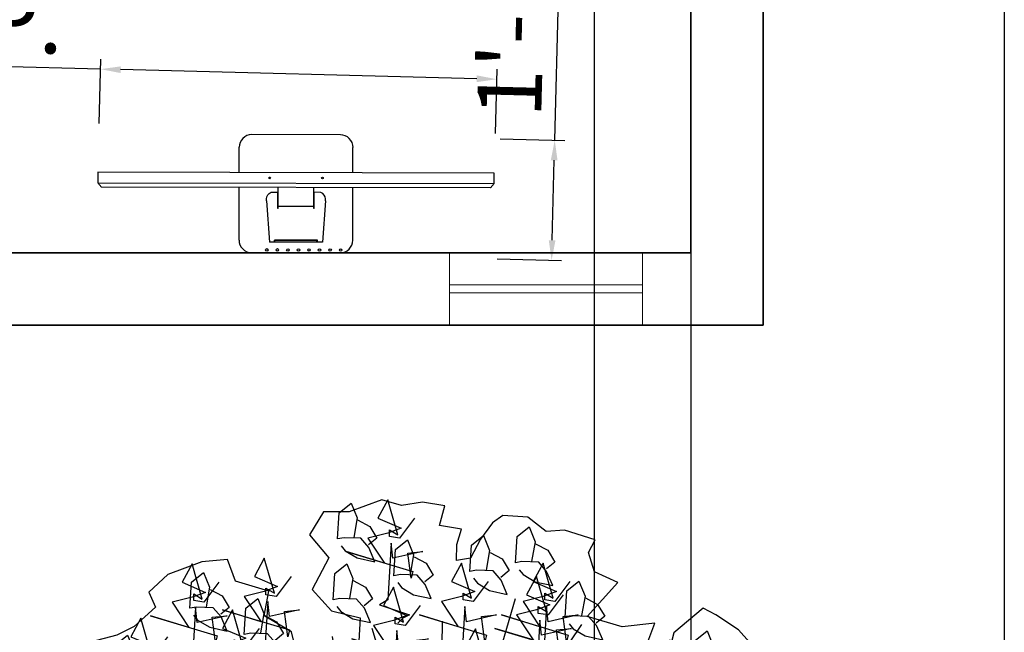
# Model space of a CAD drawing. Units: inches. Extents: x 3394 to 4794, y 965 to 1718.
# Tile 4 of 15: x 3818 to 3941, y 1160 to 1237. Entities that reach past the tile are written whole.
import ezdxf

# ---------------------------------------------------------------- set-up
doc = ezdxf.new("R2010")
doc.units = ezdxf.units.IN
for name, color, linetype, lineweight in [('A-ANNO-DIMS', 2, 'Continuous', 13), ('A-EQPM', 8, 'Continuous', 18), ('A-GLAZ', 4, 'Continuous', 18), ('A-WALL', 7, 'Continuous', 35), ('C-PROP', 7, 'Continuous', 25), ('CAY', 94, 'Continuous', 13)]:
    doc.layers.add(name, color=color, linetype=linetype, lineweight=lineweight)
for name, color, linetype in [('ARBOL', 74, 'Continuous'), ('TALLO', 36, 'Continuous'), ('window', 130, 'Continuous')]:
    doc.layers.add(name, color=color, linetype=linetype)
doc.styles.get("Standard").update_dxf_attribs({"font": 'arial.ttf'})
doc.dimstyles.new('ISO-25', dxfattribs={"dimtxt": 8, "dimasz": 2.5, "dimexe": 1.25, "dimexo": 0.625, "dimtad": 1, "dimlunit": 3, "dimtxsty": 'Standard', "dimcen": 2.5, "dimadec": 0, "dimazin": 0, "dimtfac": 1, "dimtmove": 0, "dimatfit": 3, "dimfxl": 1, "dimarcsym": 0})

# ---------------------------------------------------------------- blocks, each defined once
blk = doc.blocks.new('TV')
at = {"color": 0}
for p, q in [((3967.269, 1784.848), (3967.048, 1784.654)), ((3967.765, 1763.677), (3967.535, 1763.861))]:
    blk.add_line(p, q, dxfattribs=at)
at = {"layer": 'window'}
for p, q in [((3967.535, 1763.861), (3967.048, 1784.654)), ((3964.405, 1777.232), (3967.221, 1777.298)), ((3968.009, 1777.316), (3969.36, 1777.348)), ((3966.535, 1775.819), (3964.331, 1775.605)), ((3964.337, 1775.337), (3964.45, 1775.34)), ((3964.337, 1775.315), (3964.428, 1775.317)), ((3966.143, 1775.199), (3967.01, 1775.22)), ((3966.144, 1775.177), (3966.143, 1775.199)), ((3966.144, 1775.177), (3967.27, 1775.203)), ((3966.3, 1773.288), (3966.256, 1775.179)), ((3964.39, 1773.063), (3964.48, 1773.065)), ((3966.188, 1773.285), (3967.314, 1773.311)), ((3966.188, 1773.262), (3966.188, 1773.285)), ((3966.188, 1773.262), (3967.055, 1773.283)), ((3964.391, 1773.04), (3964.503, 1773.043)), ((3966.608, 1772.662), (3964.397, 1772.772)), ((3964.548, 1771.151), (3967.363, 1771.217)), ((3968.151, 1771.235), (3969.503, 1771.267))]:
    blk.add_line(p, q, dxfattribs=at)
for points in [[(3968.328, 1763.69), (3967.832, 1784.861), (3967.269, 1784.848), (3967.765, 1763.677), (3968.328, 1763.69)], [(3963.856, 1771.811), (3963.745, 1776.54)], [(3970.163, 1771.958), (3970.052, 1776.688)], [(3964.397, 1772.772), (3964.331, 1775.605)], [(3964.48, 1773.065), (3964.428, 1775.317)], [(3964.503, 1773.043), (3964.45, 1775.34)]]:
    blk.add_lwpolyline(points, dxfattribs=at)
for points in [[(3966.535, 1775.819, -0.263666), (3966.933, 1775.689), (3967.001, 1775.572), (3967.01, 1775.22)], [(3966.608, 1772.662, 0.263666), (3967, 1772.811), (3967.063, 1772.93), (3967.055, 1773.283)]]:
    blk.add_lwpolyline(points, format="xyb", dxfattribs=at)
for centre, radius in [((3963.914, 1775.731), 0.0679), ((3967.766, 1775.678), 0.0451), ((3963.927, 1775.168), 0.0679), ((3963.94, 1774.605), 0.0679), ((3963.953, 1774.042), 0.0679), ((3963.966, 1773.478), 0.0679), ((3963.979, 1772.915), 0.0679), ((3967.832, 1772.86), 0.0451), ((3963.993, 1772.352), 0.0679), ((3964.006, 1771.789), 0.0679)]:
    blk.add_circle(centre, radius, dxfattribs=at)
for centre, start, end in [((3969.376, 1776.672), 1.3414, 91.3414), ((3964.421, 1776.556), 91.3414, 181.3414), ((3964.532, 1771.826), 181.3414, 271.3414), ((3969.487, 1771.942), 271.3414, 1.3414)]:
    blk.add_arc(centre, 0.676, start, end, dxfattribs=at)
blk = doc.blocks.new('fresno')
at = {"layer": 'ARBOL'}
for p, q in [((2.96, 0.991), (3.575, 1.984)), ((-3.638, 1.194), (-4.164, 1.76)), ((-1.151, -0.932), (-1.99, -1.556)), ((-0.974, -3.757), (-1.31, -4.423))]:
    blk.add_line(p, q, dxfattribs=at)
blk.add_lwpolyline([(0.823, 4.745), (0.566, 4.764), (0.459, 4.687), (0.336, 4.518), (0.233, 4.322), (0.087, 4.298), (0.091, 4.464), (0.14, 4.621), (-0.09, 4.659), (-0.033, 4.863), (-0.264, 4.901), (-0.483, 4.866), (-0.686, 4.924), (-1.021, 4.801), (-1.288, 4.8), (-1.431, 4.563), (-1.234, 4.327), (-1.406, 4), (-1.205, 3.778), (-0.909, 3.705), (-0.931, 3.283), (-1.122, 2.983), (-1.491, 3.043), (-1.619, 3.562), (-1.9, 3.727), (-1.851, 3.982), (-2.197, 4.084), (-2.278, 4.31), (-2.543, 4.283), (-2.896, 4.152), (-3.091, 3.971), (-3.022, 3.817), (-3.244, 3.617), (-3.424, 3.528), (-3.697, 3.455), (-3.946, 3.236), (-3.922, 3.09), (-3.94, 2.548), (-3.617, 2.495), (-3.927, 2.19), (-4.062, 2.379), (-4.443, 2.512), (-4.546, 2.316), (-4.73, 2.062), (-4.767, 1.832), (-4.671, 1.698), (-4.486, 1.667), (-4.693, 1.559), (-4.854, 1.444), (-4.934, 1.102), (-5.037, 0.905), (-5.175, 0.644), (-5.166, 0.406), (-5.024, 0.264), (-4.781, 0.153), (-4.363, 0.249), (-4.014, 0.215), (-3.783, 0.177), (-3.46, 0.124), (-3.733, 0.051), (-4.132, -0.073), (-4.404, -0.146), (-4.639, 0.011), (-4.977, -0.028), (-5.172, -0.209), (-5.113, -0.574), (-4.921, -0.843), (-4.951, -1.027), (-5.012, -1.112), (-4.95, -1.311), (-4.83, -1.592), (-4.676, -1.807), (-4.518, -1.856), (-4.529, -2.068), (-4.417, -2.394), (-4.236, -2.59), (-4.143, -2.605), (-3.967, -2.397), (-3.703, -2.37), (-3.339, -2.027), (-3.032, -1.889), (-3.169, -2.15), (-3.115, -2.396), (-3.376, -2.542), (-3.552, -2.466), (-3.909, -2.762), (-4.077, -2.924), (-3.804, -3.135), (-3.592, -3.43), (-3.461, -3.499), (-3.253, -3.676), (-2.953, -3.867), (-2.792, -3.752), (-2.642, -3.848), (-2.572, -4.001), (-2.323, -4.066), (-2.18, -4.208), (-1.926, -4.392), (-1.58, -4.591), (-1.288, -4.545), (-1.027, -4.683), (-0.788, -4.675), (-0.531, -4.693), (-0.382, -4.505), (-0.29, -4.236), (-0.66, -3.891), (-0.588, -3.595), (-0.374, -3.441), (-0.267, -3.079), (-0.368, -2.541), (-0.208, -2.426), (-0.099, -2.633), (-0.087, -2.991), (0.071, -3.04), (0.129, -3.405), (-0.185, -3.59), (-0.119, -3.909), (0.055, -4.151), (0.136, -4.377), (0.456, -4.596), (0.828, -4.491), (1.227, -4.368), (1.461, -4.241), (1.583, -4.071), (1.748, -4.075), (1.86, -4.117), (2.101, -3.944), (2.308, -3.836), (2.925, -3.393), (3.101, -3.185), (2.74, -3.078), (2.812, -2.782), (2.769, -2.61), (3.015, -2.555), (3.012, -2.721), (3.254, -2.832), (3.546, -2.785), (3.752, -2.393), (3.882, -2.177), (3.92, -1.947), (4.069, -1.758), (4.214, -1.451), (4.144, -1.297), (4.021, -1.182), (4.182, -1.067), (4.304, -0.897), (4.464, -0.497), (4.429, -0.279), (4.406, -0.133), (3.964, -0.083), (3.074, -0.315), (2.582, -0.424), (2.217, -0.197), (2.136, 0.029), (2.462, 0.141), (2.628, -0.147), (3.012, -0.116), (3.249, 0.177), (3.602, 0.308), (3.701, 0.623), (4.089, 0.535), (4.404, 0.436), (4.464, 0.805), (4.272, 1.074), (4.267, 1.193), (4.336, 1.324), (4.243, 1.623), (4.092, 2.003), (3.769, 2.057), (3.485, 2.056), (3.642, 2.291), (3.88, 2.299), (3.71, 2.706), (3.563, 2.967), (3.201, 3.358), (3.001, 3.581), (2.766, 3.738), (2.635, 3.807), (2.332, 3.549), (2.268, 3.299), (2.052, 3.429), (2.136, 3.652), (1.798, 3.613), (1.437, 3.72), (1.755, 4.071), (1.513, 4.182), (1.451, 4.381), (1.519, 4.512), (1.204, 4.611), (1.012, 4.596)], close=True, dxfattribs=at)
for points in [[(-1.104, 4.45), (-1.063, 4.399), (-0.939, 4.325), (-0.757, 4.285), (-0.82, 4.431), (-0.903, 4.527), (-1.075, 4.533), (-1.143, 4.521), (-1.126, 4.792), (-1.002, 4.891), (-0.939, 4.738), (-0.975, 4.535)], [(-0.346, 4.735), (-0.501, 4.528), (-0.605, 4.545), (-0.605, 4.614), (-0.519, 4.563), (-0.622, 4.925), (-0.726, 4.735), (-0.484, 4.632), (-0.622, 4.58), (-0.829, 4.528), (-0.657, 4.27), (-1.053, 4.39), (-0.363, 4.183), (-0.381, 4.114), (-0.415, 4.373), (-0.26, 4.39), (-0.57, 4.321), (-0.588, 4.476), (-0.622, 3.89), (-0.708, 3.839), (-0.398, 3.735), (-0.467, 3.701), (-0.519, 3.649)], [(-0.935, 4.717), (-0.809, 4.65), (-0.736, 4.529), (-0.824, 4.459)], [(0.734, 4.203), (0.775, 4.152), (0.9, 4.078), (1.082, 4.038), (1.018, 4.185), (0.936, 4.281), (0.763, 4.287), (0.696, 4.274), (0.712, 4.546), (0.837, 4.645), (0.899, 4.491), (0.863, 4.289)], [(-0.521, 4.069), (-0.48, 4.018), (-0.356, 3.944), (-0.174, 3.904), (-0.237, 4.051), (-0.32, 4.146), (-0.492, 4.152), (-0.56, 4.14), (-0.543, 4.411), (-0.419, 4.511), (-0.356, 4.357), (-0.392, 4.154)], [(0.263, 4.114), (0.304, 4.063), (0.429, 3.989), (0.611, 3.948), (0.547, 4.095), (0.465, 4.191), (0.293, 4.197), (0.225, 4.185), (0.242, 4.456), (0.366, 4.555), (0.428, 4.402), (0.393, 4.199)], [(0.433, 4.381), (0.558, 4.314), (0.631, 4.193), (0.544, 4.122)], [(0.904, 4.471), (1.029, 4.404), (1.102, 4.282), (1.015, 4.212)], [(-1.623, 4.132), (-1.778, 3.925), (-1.882, 3.942), (-1.882, 4.011), (-1.795, 3.959), (-1.899, 4.321), (-2.002, 4.132), (-1.761, 4.028), (-1.899, 3.977), (-2.106, 3.925), (-1.933, 3.666), (-2.33, 3.787), (-1.64, 3.58), (-1.657, 3.511), (-1.692, 3.77), (-1.537, 3.787), (-1.847, 3.718), (-1.864, 3.873), (-1.899, 3.287), (-1.985, 3.235), (-1.675, 3.132), (-1.744, 3.097), (-1.795, 3.046)], [(-0.352, 4.337), (-0.226, 4.269), (-0.153, 4.148), (-0.241, 4.078)], [(-2.368, 4.073), (-2.523, 3.866), (-2.627, 3.883), (-2.627, 3.952), (-2.541, 3.9), (-2.644, 4.262), (-2.748, 4.073), (-2.506, 3.969), (-2.644, 3.918), (-2.851, 3.866), (-2.679, 3.607), (-3.075, 3.728), (-2.385, 3.521), (-2.403, 3.452), (-2.437, 3.711), (-2.282, 3.728), (-2.592, 3.659), (-2.61, 3.814), (-2.644, 3.228), (-2.73, 3.176), (-2.42, 3.073), (-2.489, 3.038), (-2.541, 2.987)], [(-2.629, 3.733), (-2.588, 3.682), (-2.463, 3.608), (-2.281, 3.568), (-2.345, 3.715), (-2.427, 3.81), (-2.6, 3.816), (-2.667, 3.804), (-2.651, 4.075), (-2.526, 4.175), (-2.464, 4.021), (-2.5, 3.818)], [(-1.149, 3.822), (-1.108, 3.771), (-0.983, 3.697), (-0.802, 3.657), (-0.865, 3.804), (-0.948, 3.9), (-1.12, 3.906), (-1.188, 3.893), (-1.171, 4.165), (-1.047, 4.264), (-0.984, 4.111), (-1.02, 3.908)], [(0.413, 4.08), (0.258, 3.873), (0.154, 3.89), (0.154, 3.959), (0.241, 3.908), (0.137, 4.27), (0.034, 4.08), (0.275, 3.977), (0.137, 3.925), (-0.07, 3.873), (0.103, 3.614), (-0.294, 3.735), (0.396, 3.528), (0.379, 3.459), (0.344, 3.718), (0.499, 3.735), (0.189, 3.666), (0.172, 3.821), (0.137, 3.235), (0.051, 3.183), (0.361, 3.08), (0.292, 3.046), (0.241, 2.994)], [(1.259, 4.08), (1.103, 3.873), (1, 3.89), (1, 3.959), (1.086, 3.908), (0.982, 4.27), (0.879, 4.08), (1.12, 3.977), (0.982, 3.925), (0.775, 3.873), (0.948, 3.614), (0.551, 3.735), (1.241, 3.528), (1.224, 3.459), (1.189, 3.718), (1.345, 3.735), (1.034, 3.666), (1.017, 3.821), (0.982, 3.235), (0.896, 3.183), (1.207, 3.08), (1.138, 3.046), (1.086, 2.994)], [(-0.98, 4.09), (-0.854, 4.023), (-0.781, 3.901), (-0.869, 3.831)], [(1.189, 3.942), (1.034, 3.735), (0.931, 3.752), (0.931, 3.821), (1.017, 3.77), (0.913, 4.132), (0.81, 3.942), (1.051, 3.839), (0.913, 3.787), (0.706, 3.735), (0.879, 3.477), (0.482, 3.597), (1.172, 3.39), (1.155, 3.321), (1.12, 3.58), (1.276, 3.597), (0.965, 3.528), (0.948, 3.683), (0.913, 3.097), (0.827, 3.046), (1.138, 2.942), (1.069, 2.908), (1.017, 2.856)], [(1.25, 3.643), (1.291, 3.592), (1.416, 3.518), (1.597, 3.478), (1.534, 3.625), (1.451, 3.721), (1.279, 3.727), (1.211, 3.714), (1.228, 3.985), (1.352, 4.085), (1.415, 3.931), (1.379, 3.729)], [(-2.459, 4), (-2.334, 3.933), (-2.261, 3.812), (-2.348, 3.742)], [(-0.287, 3.833), (-0.442, 3.626), (-0.546, 3.643), (-0.546, 3.712), (-0.46, 3.661), (-0.563, 4.023), (-0.667, 3.833), (-0.425, 3.73), (-0.563, 3.678), (-0.77, 3.626), (-0.598, 3.367), (-0.995, 3.488), (-0.304, 3.281), (-0.322, 3.212), (-0.356, 3.471), (-0.201, 3.488), (-0.511, 3.419), (-0.529, 3.574), (-0.563, 2.988), (-0.649, 2.936), (-0.339, 2.833), (-0.408, 2.799), (-0.46, 2.747)], [(-2.068, 3.464), (-2.027, 3.413), (-1.903, 3.339), (-1.721, 3.299), (-1.784, 3.446), (-1.867, 3.542), (-2.039, 3.547), (-2.107, 3.535), (-2.09, 3.806), (-1.966, 3.906), (-1.903, 3.752), (-1.939, 3.55)], [(0.837, 2.414), (0.533, 3.352), (0.697, 3.906)], [(1.419, 3.911), (1.545, 3.844), (1.618, 3.722), (1.53, 3.652)], [(-1.951, 3.597), (-2.106, 3.39), (-2.209, 3.408), (-2.209, 3.477), (-2.123, 3.425), (-2.227, 3.787), (-2.33, 3.597), (-2.089, 3.494), (-2.227, 3.442), (-2.434, 3.39), (-2.261, 3.132), (-2.658, 3.252), (-1.968, 3.046), (-1.985, 2.977), (-2.02, 3.235), (-1.864, 3.252), (-2.175, 3.183), (-2.192, 3.339), (-2.227, 2.752), (-2.313, 2.701), (-2.002, 2.597), (-2.071, 2.563), (-2.123, 2.511)], [(-2.898, 3.511), (-3.053, 3.304), (-3.157, 3.321), (-3.157, 3.39), (-3.071, 3.339), (-3.174, 3.701), (-3.278, 3.511), (-3.036, 3.408), (-3.174, 3.356), (-3.381, 3.304), (-3.209, 3.046), (-3.605, 3.166), (-2.915, 2.959), (-2.932, 2.89), (-2.967, 3.149), (-2.812, 3.166), (-3.122, 3.097), (-3.14, 3.253), (-3.174, 2.666), (-3.26, 2.615), (-2.95, 2.511), (-3.019, 2.477), (-3.071, 2.425)], [(-1.899, 3.732), (-1.773, 3.664), (-1.7, 3.543), (-1.788, 3.473)], [(-0.063, 3.671), (-0.069, 3.151), (-0.364, 2.965), (-0.319, 2.449)], [(-0.358, 2.895), (-0.615, 3.037), (-0.783, 3.596)], [(0.558, 3.402), (0.403, 3.195), (0.299, 3.212), (0.299, 3.281), (0.386, 3.23), (0.282, 3.592), (0.179, 3.402), (0.42, 3.299), (0.282, 3.247), (0.075, 3.195), (0.248, 2.936), (-0.149, 3.057), (0.541, 2.85), (0.524, 2.781), (0.489, 3.04), (0.644, 3.057), (0.334, 2.988), (0.317, 3.143), (0.282, 2.557), (0.196, 2.505), (0.506, 2.402), (0.437, 2.368), (0.386, 2.316)], [(1.259, 2.882), (1.254, 3.446), (1.381, 3.636)], [(2.573, 3.128), (2.613, 3.077), (2.738, 3.003), (2.92, 2.963), (2.857, 3.11), (2.774, 3.205), (2.602, 3.211), (2.534, 3.199), (2.551, 3.47), (2.675, 3.57), (2.738, 3.416), (2.702, 3.214)], [(-3.413, 3.083), (-3.373, 3.032), (-3.248, 2.958), (-3.066, 2.918), (-3.129, 3.065), (-3.212, 3.161), (-3.384, 3.167), (-3.452, 3.154), (-3.435, 3.425), (-3.311, 3.525), (-3.248, 3.371), (-3.284, 3.169)], [(-1.367, 2.367), (-1.081, 2.78), (-1.193, 3.514)], [(2.191, 3.038), (2.232, 2.987), (2.357, 2.913), (2.539, 2.873), (2.475, 3.02), (2.393, 3.116), (2.221, 3.122), (2.153, 3.109), (2.17, 3.381), (2.294, 3.48), (2.356, 3.326), (2.321, 3.124)], [(-0.923, 3.449), (-0.951, 3.425), (-0.93, 3.313)], [(-0.41, 3.035), (-0.387, 2.974), (-0.291, 2.865), (-0.131, 2.771), (-0.146, 2.93), (-0.195, 3.047), (-0.357, 3.106), (-0.425, 3.115), (-0.325, 3.368), (-0.176, 3.424), (-0.164, 3.258), (-0.261, 3.077)], [(0.746, 2.242), (1.034, 2.786), (1.584, 3.019), (1.879, 3.374)], [(1.564, 3.016), (1.605, 2.965), (1.729, 2.891), (1.911, 2.851), (1.848, 2.998), (1.765, 3.094), (1.593, 3.099), (1.525, 3.087), (1.542, 3.358), (1.666, 3.458), (1.729, 3.304), (1.693, 3.102)], [(2.742, 3.396), (2.868, 3.328), (2.941, 3.207), (2.853, 3.137)], [(-3.244, 3.351), (-3.118, 3.284), (-3.045, 3.162), (-3.133, 3.092)], [(-0.448, 1), (-0.961, 1.419), (-1.784, 3.341)], [(1.733, 3.284), (1.859, 3.216), (1.932, 3.095), (1.844, 3.025)], [(2.361, 3.306), (2.486, 3.239), (2.559, 3.117), (2.472, 3.047)], [(3.111, 2.904), (3.152, 2.853), (3.276, 2.779), (3.458, 2.739), (3.395, 2.886), (3.312, 2.981), (3.14, 2.987), (3.072, 2.975), (3.089, 3.246), (3.213, 3.346), (3.276, 3.192), (3.24, 2.99)], [(-2.225, 2.77), (-2.184, 2.718), (-2.06, 2.645), (-1.878, 2.604), (-1.941, 2.751), (-2.024, 2.847), (-2.196, 2.853), (-2.264, 2.84), (-2.247, 3.112), (-2.123, 3.211), (-2.06, 3.058), (-2.096, 2.855)], [(-1.575, 2.854), (-2.052, 2.969), (-2.2, 3.178)], [(-1.373, 2.77), (-1.332, 2.718), (-1.208, 2.645), (-1.026, 2.604), (-1.089, 2.751), (-1.172, 2.847), (-1.344, 2.853), (-1.412, 2.84), (-1.395, 3.112), (-1.271, 3.211), (-1.208, 3.058), (-1.244, 2.855)], [(-0.166, 3.238), (-0.068, 3.135), (-0.036, 2.997), (-0.141, 2.957)], [(3.28, 3.172), (3.406, 3.104), (3.479, 2.983), (3.391, 2.913)], [(2.326, 2.702), (2.367, 2.651), (2.492, 2.577), (2.673, 2.537), (2.61, 2.684), (2.527, 2.78), (2.355, 2.786), (2.287, 2.773), (2.304, 3.045), (2.428, 3.144), (2.491, 2.99), (2.455, 2.788)], [(-1.112, 1.773), (-2.014, 2.265), (-2.654, 2.957)], [(-2.056, 3.037), (-1.93, 2.97), (-1.857, 2.849), (-1.945, 2.778)], [(-0.57, 2.77), (-0.726, 2.563), (-0.829, 2.58), (-0.829, 2.649), (-0.743, 2.597), (-0.846, 2.959), (-0.95, 2.77), (-0.708, 2.666), (-0.846, 2.615), (-1.053, 2.563), (-0.881, 2.304), (-1.278, 2.425), (-0.588, 2.218), (-0.605, 2.149), (-0.639, 2.408), (-0.484, 2.425), (-0.795, 2.356), (-0.812, 2.511), (-0.846, 1.925), (-0.933, 1.873), (-0.622, 1.77), (-0.691, 1.735), (-0.743, 1.684)], [(-1.204, 3.037), (-1.078, 2.97), (-1.005, 2.849), (-1.093, 2.778)], [(2.121, 2.804), (1.966, 2.597), (1.862, 2.615), (1.862, 2.683), (1.949, 2.632), (1.845, 2.994), (1.742, 2.804), (1.983, 2.701), (1.845, 2.649), (1.638, 2.597), (1.811, 2.339), (1.414, 2.459), (2.104, 2.252), (2.087, 2.184), (2.052, 2.442), (2.207, 2.459), (1.897, 2.39), (1.88, 2.546), (1.845, 1.959), (1.759, 1.908), (2.069, 1.804), (2, 1.77), (1.949, 1.718)], [(2.495, 2.97), (2.621, 2.903), (2.694, 2.781), (2.606, 2.711)], [(-3.434, 2.752), (-3.59, 2.546), (-3.693, 2.563), (-3.693, 2.632), (-3.607, 2.58), (-3.71, 2.942), (-3.814, 2.752), (-3.572, 2.649), (-3.71, 2.597), (-3.917, 2.546), (-3.745, 2.287), (-4.142, 2.408), (-3.452, 2.201), (-3.469, 2.132), (-3.503, 2.39), (-3.348, 2.408), (-3.659, 2.339), (-3.676, 2.494), (-3.71, 1.908), (-3.797, 1.856), (-3.486, 1.753), (-3.555, 1.718), (-3.607, 1.666)], [(2.171, 1.674), (2.121, 2.172), (2.689, 2.898)], [(3.519, 2.666), (3.363, 2.459), (3.26, 2.477), (3.26, 2.546), (3.346, 2.494), (3.243, 2.856), (3.139, 2.666), (3.381, 2.563), (3.243, 2.511), (3.036, 2.459), (3.208, 2.201), (2.811, 2.321), (3.501, 2.115), (3.484, 2.046), (3.45, 2.304), (3.605, 2.321), (3.294, 2.252), (3.277, 2.408), (3.243, 1.821), (3.156, 1.77), (3.467, 1.666), (3.398, 1.632), (3.346, 1.58)], [(3.043, 2.478), (3.084, 2.427), (3.209, 2.353), (3.391, 2.313), (3.327, 2.46), (3.245, 2.556), (3.073, 2.562), (3.005, 2.549), (3.022, 2.82), (3.146, 2.92), (3.208, 2.766), (3.173, 2.564)], [(1.586, 2.528), (1.431, 2.321), (1.327, 2.339), (1.327, 2.408), (1.414, 2.356), (1.31, 2.718), (1.207, 2.528), (1.448, 2.425), (1.31, 2.373), (1.103, 2.321), (1.276, 2.063), (0.879, 2.184), (1.569, 1.977), (1.552, 1.908), (1.517, 2.166), (1.673, 2.184), (1.362, 2.115), (1.345, 2.27), (1.31, 1.684), (1.224, 1.632), (1.535, 1.528), (1.466, 1.494), (1.414, 1.442)], [(3.213, 2.746), (3.338, 2.679), (3.411, 2.557), (3.324, 2.487)], [(3.178, 2.165), (3.219, 2.113), (3.344, 2.04), (3.525, 1.999), (3.462, 2.146), (3.379, 2.242), (3.207, 2.248), (3.139, 2.236), (3.156, 2.507), (3.28, 2.606), (3.343, 2.453), (3.307, 2.25)], [(-4.422, 2.03), (-4.381, 1.979), (-4.257, 1.905), (-4.075, 1.865), (-4.138, 2.012), (-4.221, 2.108), (-4.393, 2.114), (-4.461, 2.101), (-4.444, 2.372), (-4.32, 2.472), (-4.257, 2.318), (-4.293, 2.116)], [(-3.468, 1.85), (-3.409, 2.222), (-3.628, 2.505)], [(-1.817, 2.351), (-1.972, 2.144), (-2.075, 2.162), (-2.075, 2.231), (-1.989, 2.179), (-2.093, 2.541), (-2.196, 2.351), (-1.955, 2.248), (-2.093, 2.196), (-2.3, 2.144), (-2.127, 1.886), (-2.524, 2.006), (-1.834, 1.8), (-1.851, 1.731), (-1.886, 1.989), (-1.73, 2.006), (-2.041, 1.937), (-2.058, 2.093), (-2.093, 1.506), (-2.179, 1.455), (-1.868, 1.351), (-1.937, 1.317), (-1.989, 1.265)], [(-1.786, 2.007), (-1.722, 1.99), (-1.578, 2.003), (-1.407, 2.078), (-1.545, 2.159), (-1.668, 2.188), (-1.811, 2.092), (-1.859, 2.042), (-2.004, 2.271), (-1.962, 2.425), (-1.821, 2.337), (-1.731, 2.152)], [(-1.806, 2.323), (-1.665, 2.343), (-1.534, 2.287), (-1.564, 2.179)], [(3.245, 1.963), (3.286, 1.912), (3.411, 1.838), (3.593, 1.798), (3.529, 1.945), (3.447, 2.041), (3.274, 2.046), (3.206, 2.034), (3.223, 2.305), (3.347, 2.405), (3.41, 2.251), (3.374, 2.049)], [(3.347, 2.432), (3.473, 2.365), (3.546, 2.244), (3.458, 2.173)], [(-3.986, 2.149), (-4.142, 1.942), (-4.245, 1.959), (-4.245, 2.028), (-4.159, 1.977), (-4.262, 2.339), (-4.366, 2.149), (-4.124, 2.046), (-4.262, 1.994), (-4.47, 1.942), (-4.297, 1.684), (-4.694, 1.804), (-4.004, 1.597), (-4.021, 1.528), (-4.055, 1.787), (-3.9, 1.804), (-4.211, 1.735), (-4.228, 1.89), (-4.262, 1.304), (-4.349, 1.253), (-4.038, 1.149), (-4.107, 1.115), (-4.159, 1.063)], [(-4.253, 2.298), (-4.127, 2.231), (-4.054, 2.109), (-4.142, 2.039)], [(-3.533, 2.149), (-3.43, 2.247), (-3.292, 2.279), (-3.252, 2.174)], [(-0.566, 1.873), (-0.525, 1.822), (-0.4, 1.748), (-0.219, 1.708), (-0.282, 1.855), (-0.365, 1.951), (-0.537, 1.957), (-0.605, 1.944), (-0.588, 2.216), (-0.464, 2.315), (-0.401, 2.162), (-0.437, 1.959)], [(-2.916, 0.958), (-3.096, 1.528), (-3.871, 2.197)], [(-3.331, 1.905), (-3.269, 1.928), (-3.161, 2.024), (-3.066, 2.184), (-3.226, 2.169), (-3.342, 2.121), (-3.401, 1.958), (-3.41, 1.89), (-3.663, 1.99), (-3.719, 2.139), (-3.554, 2.151), (-3.372, 2.054)], [(-0.397, 2.141), (-0.271, 2.074), (-0.198, 1.952), (-0.286, 1.882)], [(3.415, 2.231), (3.54, 2.163), (3.613, 2.042), (3.525, 1.972)], [(-1.164, 1.612), (-1.109, 1.576), (-0.967, 1.544), (-0.782, 1.562), (-0.888, 1.682), (-0.996, 1.748), (-1.162, 1.7), (-1.222, 1.667), (-1.29, 1.93), (-1.203, 2.063), (-1.096, 1.937), (-1.067, 1.733)], [(0.72, 1.798), (0.723, 1.733), (0.781, 1.6), (0.904, 1.46), (0.939, 1.616), (0.929, 1.742), (0.793, 1.848), (0.73, 1.878), (0.904, 2.088), (1.062, 2.095), (1.023, 1.934), (0.875, 1.791)], [(-2.965, 1.493), (-2.924, 1.441), (-2.799, 1.368), (-2.618, 1.327), (-2.681, 1.474), (-2.764, 1.57), (-2.936, 1.576), (-3.004, 1.564), (-2.987, 1.835), (-2.863, 1.934), (-2.8, 1.781), (-2.836, 1.578)], [(3.649, 1.515), (3.69, 1.464), (3.814, 1.39), (3.996, 1.35), (3.933, 1.497), (3.85, 1.592), (3.678, 1.598), (3.61, 1.586), (3.627, 1.857), (3.751, 1.957), (3.814, 1.803), (3.778, 1.601)], [(3.716, 1.537), (3.757, 1.486), (3.882, 1.412), (4.063, 1.372), (4, 1.519), (3.917, 1.615), (3.745, 1.621), (3.677, 1.608), (3.694, 1.88), (3.818, 1.979), (3.881, 1.825), (3.845, 1.623)], [(-1.085, 1.919), (-0.945, 1.893), (-0.838, 1.801), (-0.9, 1.707)], [(1.014, 1.915), (1.077, 1.787), (1.064, 1.646), (0.952, 1.64)], [(2.587, 1.684), (2.432, 1.477), (2.328, 1.494), (2.328, 1.563), (2.414, 1.511), (2.311, 1.873), (2.207, 1.684), (2.449, 1.58), (2.311, 1.528), (2.104, 1.477), (2.276, 1.218), (1.88, 1.339), (2.57, 1.132), (2.552, 1.063), (2.518, 1.321), (2.673, 1.339), (2.363, 1.27), (2.345, 1.425), (2.311, 0.839), (2.225, 0.787), (2.535, 0.684), (2.466, 0.649), (2.414, 0.597)], [(-2.796, 1.76), (-2.67, 1.693), (-2.597, 1.572), (-2.685, 1.501)], [(3.818, 1.783), (3.944, 1.715), (4.017, 1.594), (3.929, 1.524)], [(3.885, 1.805), (4.011, 1.738), (4.084, 1.616), (3.996, 1.546)], [(-4.759, 1.269), (-4.718, 1.217), (-4.593, 1.144), (-4.411, 1.103), (-4.475, 1.25), (-4.557, 1.346), (-4.729, 1.352), (-4.797, 1.339), (-4.78, 1.611), (-4.656, 1.71), (-4.594, 1.557), (-4.629, 1.354)], [(-1.575, 1.269), (-1.534, 1.217), (-1.409, 1.144), (-1.228, 1.103), (-1.291, 1.25), (-1.373, 1.346), (-1.546, 1.352), (-1.614, 1.339), (-1.597, 1.611), (-1.473, 1.71), (-1.41, 1.557), (-1.446, 1.354)], [(1.283, 1.469), (1.266, 1.405), (1.279, 1.261), (1.354, 1.09), (1.435, 1.228), (1.464, 1.351), (1.368, 1.494), (1.318, 1.542), (1.547, 1.687), (1.7, 1.645), (1.613, 1.504), (1.428, 1.414)], [(-4.193, 1.356), (-4.349, 1.149), (-4.452, 1.166), (-4.452, 1.235), (-4.366, 1.184), (-4.469, 1.546), (-4.573, 1.356), (-4.331, 1.253), (-4.469, 1.201), (-4.677, 1.149), (-4.504, 0.89), (-4.901, 1.011), (-4.211, 0.804), (-4.228, 0.735), (-4.262, 0.994), (-4.107, 1.011), (-4.418, 0.942), (-4.435, 1.097), (-4.469, 0.511), (-4.556, 0.459), (-4.245, 0.356), (-4.314, 0.322), (-4.366, 0.27)], [(-4.589, 1.536), (-4.464, 1.469), (-4.391, 1.348), (-4.478, 1.277)], [(-1.406, 1.536), (-1.28, 1.469), (-1.207, 1.348), (-1.295, 1.277)], [(3.761, 1.112), (3.802, 1.061), (3.926, 0.987), (4.108, 0.947), (4.045, 1.093), (3.962, 1.189), (3.79, 1.195), (3.722, 1.183), (3.739, 1.454), (3.863, 1.553), (3.926, 1.4), (3.89, 1.197)], [(1.599, 1.489), (1.618, 1.348), (1.563, 1.217), (1.455, 1.247)], [(2.479, 1.34), (2.443, 1.285), (2.411, 1.143), (2.429, 0.958), (2.549, 1.064), (2.615, 1.172), (2.567, 1.338), (2.534, 1.398), (2.797, 1.466), (2.93, 1.379), (2.804, 1.272), (2.6, 1.243)], [(3.139, 1.235), (2.984, 1.028), (2.88, 1.046), (2.88, 1.115), (2.967, 1.063), (2.863, 1.425), (2.759, 1.235), (3.001, 1.132), (2.863, 1.08), (2.656, 1.028), (2.828, 0.77), (2.432, 0.891), (3.122, 0.684), (3.105, 0.615), (3.07, 0.873), (3.225, 0.891), (2.915, 0.822), (2.897, 0.977), (2.863, 0.391), (2.777, 0.339), (3.087, 0.235), (3.018, 0.201), (2.967, 0.149)], [(-3.192, 1.017), (-3.578, 1.215), (-3.949, 1.081), (-4.398, 1.339)], [(0.308, 0.933), (0.349, 0.881), (0.474, 0.807), (0.656, 0.767), (0.592, 0.914), (0.51, 1.01), (0.337, 1.016), (0.27, 1.003), (0.286, 1.275), (0.411, 1.374), (0.473, 1.221), (0.437, 1.018)], [(4.01, 1.36), (3.422, 0.918)], [(3.93, 1.379), (4.056, 1.312), (4.129, 1.191), (4.041, 1.121)], [(-3.481, 0.843), (-3.44, 0.792), (-3.315, 0.718), (-3.133, 0.678), (-3.197, 0.825), (-3.279, 0.92), (-3.451, 0.926), (-3.519, 0.914), (-3.502, 1.185), (-3.378, 1.285), (-3.316, 1.131), (-3.351, 0.928)], [(-2.703, 1.201), (-2.575, 1.263), (-2.433, 1.251), (-2.428, 1.139)], [(2.786, 1.261), (2.76, 1.121), (2.668, 1.014), (2.574, 1.076)], [(4.26, 1.115), (4.105, 0.908), (4.002, 0.925), (4.002, 0.994), (4.088, 0.942), (3.984, 1.304), (3.881, 1.115), (4.122, 1.011), (3.984, 0.959), (3.777, 0.908), (3.95, 0.649), (3.553, 0.77), (4.243, 0.563), (4.226, 0.494), (4.191, 0.753), (4.347, 0.77), (4.036, 0.701), (4.019, 0.856), (3.984, 0.27), (3.898, 0.218), (4.209, 0.115), (4.14, 0.08), (4.088, 0.029)], [(-3.354, 1.176), (-4.529, 0.864)], [(0.478, 1.2), (0.603, 1.133), (0.676, 1.011), (0.589, 0.941)], [(-3.311, 1.111), (-3.186, 1.043), (-3.113, 0.922), (-3.2, 0.852)], [(2.808, 1.015), (3.422, 0.918), (3.422, 0.918), (3.748, 0.794), (4.154, 1.111)], [(-1.981, 0.615), (-1.915, 0.618), (-1.782, 0.676), (-1.643, 0.799), (-1.799, 0.834), (-1.925, 0.824), (-2.031, 0.688), (-2.061, 0.626), (-2.27, 0.799), (-2.278, 0.958), (-2.117, 0.918), (-1.974, 0.77)], [(4.075, 0.529), (4.116, 0.478), (4.24, 0.404), (4.422, 0.364), (4.359, 0.511), (4.276, 0.607), (4.104, 0.613), (4.036, 0.6), (4.053, 0.871), (4.177, 0.971), (4.24, 0.817), (4.204, 0.615)], [(-5.028, 0.44), (-4.987, 0.388), (-4.862, 0.315), (-4.68, 0.274), (-4.744, 0.421), (-4.826, 0.517), (-4.998, 0.523), (-5.066, 0.511), (-5.049, 0.782), (-4.925, 0.881), (-4.863, 0.728), (-4.898, 0.525)], [(-0.397, 0.517), (-0.346, 0.557), (-0.272, 0.682), (-0.232, 0.864), (-0.379, 0.801), (-0.474, 0.718), (-0.48, 0.546), (-0.468, 0.478), (-0.739, 0.495), (-0.838, 0.619), (-0.685, 0.682), (-0.482, 0.646)], [(-4.602, 0.35), (-4.561, 0.299), (-4.436, 0.225), (-4.254, 0.185), (-4.318, 0.332), (-4.4, 0.428), (-4.572, 0.433), (-4.64, 0.421), (-4.623, 0.692), (-4.499, 0.792), (-4.437, 0.638), (-4.472, 0.436)], [(2.639, 0.58), (2.483, 0.373), (2.38, 0.391), (2.38, 0.46), (2.466, 0.408), (2.363, 0.77), (2.259, 0.58), (2.501, 0.477), (2.363, 0.425), (2.156, 0.373), (2.328, 0.115), (1.931, 0.235), (2.621, 0.029), (2.604, -0.04), (2.57, 0.218), (2.725, 0.235), (2.414, 0.166), (2.397, 0.322), (2.363, -0.265), (2.276, -0.316), (2.587, -0.42), (2.518, -0.454), (2.466, -0.506)], [(2.708, 0.563), (2.552, 0.356), (2.449, 0.373), (2.449, 0.442), (2.535, 0.391), (2.432, 0.753), (2.328, 0.563), (2.57, 0.46), (2.432, 0.408), (2.225, 0.356), (2.397, 0.097), (2, 0.218), (2.69, 0.011), (2.673, -0.058), (2.639, 0.201), (2.794, 0.218), (2.483, 0.149), (2.466, 0.304), (2.432, -0.282), (2.345, -0.334), (2.656, -0.437), (2.587, -0.471), (2.535, -0.523)], [(4.244, 0.797), (4.37, 0.73), (4.443, 0.608), (4.355, 0.538)], [(-4.858, 0.707), (-4.733, 0.64), (-4.66, 0.519), (-4.747, 0.448)], [(-4.432, 0.618), (-4.307, 0.55), (-4.234, 0.429), (-4.321, 0.359)], [(-3.824, 0.404), (-3.763, 0.427), (-3.654, 0.523), (-3.559, 0.683), (-3.719, 0.668), (-3.835, 0.62), (-3.894, 0.457), (-3.903, 0.389), (-4.156, 0.489), (-4.212, 0.638), (-4.047, 0.65), (-3.865, 0.553)], [(-2.698, 0.509), (-2.854, 0.302), (-2.957, 0.319), (-2.957, 0.388), (-2.871, 0.336), (-2.974, 0.698), (-3.078, 0.509), (-2.836, 0.405), (-2.974, 0.353), (-3.182, 0.302), (-3.009, 0.043), (-3.406, 0.164), (-2.716, -0.043), (-2.733, -0.112), (-2.767, 0.147), (-2.612, 0.164), (-2.923, 0.095), (-2.94, 0.25), (-2.974, -0.336), (-3.061, -0.388), (-2.75, -0.491), (-2.819, -0.526), (-2.871, -0.577)], [(1.978, 0.384), (1.927, 0.343), (1.853, 0.218), (1.813, 0.036), (1.96, 0.1), (2.056, 0.182), (2.061, 0.355), (2.049, 0.422), (2.32, 0.406), (2.42, 0.281), (2.266, 0.219), (2.064, 0.254)], [(-2.322, 0.222), (-2.219, 0.321), (-2.081, 0.353), (-2.042, 0.248)], [(3.829, 0.184), (3.674, -0.023), (3.57, -0.006), (3.57, 0.063), (3.657, 0.011), (3.553, 0.373), (3.45, 0.184), (3.691, 0.08), (3.553, 0.029), (3.346, -0.023), (3.519, -0.282), (3.122, -0.161), (3.812, -0.368), (3.795, -0.437), (3.76, -0.178), (3.915, -0.161), (3.605, -0.23), (3.588, -0.075), (3.553, -0.661), (3.467, -0.713), (3.777, -0.816), (3.708, -0.851), (3.657, -0.902)], [(-3.394, 0.18), (-3.77, 0.182), (-4.532, 0.27)], [(-0.596, -0.564), (0.03, -0.026), (0.339, 0.235)], [(2.246, 0.214), (2.178, 0.089), (2.057, 0.016), (1.987, 0.103)], [(-3.77, 0.182), (-4.09, -0.088), (-4.494, -0.18)], [(0.03, -0.026), (-0.491, 0.154), (-0.871, -0.08)], [(0.38, 0.131), (0.248, -0.21), (-0.33, -0.951)], [(-1.642, -0.412), (-1.601, -0.463), (-1.477, -0.537), (-1.295, -0.577), (-1.358, -0.43), (-1.441, -0.334), (-1.613, -0.328), (-1.681, -0.341), (-1.664, -0.069), (-1.54, 0.03), (-1.477, -0.124), (-1.513, -0.326)], [(-4.871, -0.524), (-4.83, -0.575), (-4.705, -0.649), (-4.523, -0.689), (-4.587, -0.542), (-4.669, -0.446), (-4.841, -0.44), (-4.909, -0.453), (-4.893, -0.181), (-4.768, -0.082), (-4.706, -0.236), (-4.741, -0.438)], [(3.139, -0.282), (2.984, -0.489), (2.88, -0.471), (2.88, -0.402), (2.967, -0.454), (2.863, -0.092), (2.759, -0.282), (3.001, -0.385), (2.863, -0.437), (2.656, -0.489), (2.828, -0.747), (2.432, -0.627), (3.122, -0.834), (3.105, -0.902), (3.07, -0.644), (3.225, -0.627), (2.915, -0.696), (2.897, -0.54), (2.863, -1.127), (2.777, -1.178), (3.087, -1.282), (3.018, -1.316), (2.967, -1.368)], [(-3.848, -0.389), (-3.781, -0.264), (-3.659, -0.191), (-3.589, -0.278)], [(-1.473, -0.144), (-1.347, -0.211), (-1.274, -0.333), (-1.362, -0.403)], [(-4.701, -0.256), (-4.576, -0.323), (-4.503, -0.445), (-4.59, -0.515)], [(-3.952, -0.42), (-4.107, -0.627), (-4.211, -0.609), (-4.211, -0.54), (-4.124, -0.592), (-4.228, -0.23), (-4.331, -0.42), (-4.09, -0.523), (-4.228, -0.575), (-4.435, -0.627), (-4.262, -0.885), (-4.659, -0.765), (-3.969, -0.971), (-3.986, -1.04), (-4.021, -0.782), (-3.866, -0.765), (-4.176, -0.834), (-4.193, -0.678), (-4.228, -1.265), (-4.314, -1.316), (-4.004, -1.42), (-4.073, -1.454), (-4.124, -1.506)], [(-3.58, -0.559), (-3.529, -0.518), (-3.455, -0.393), (-3.415, -0.211), (-3.562, -0.275), (-3.658, -0.357), (-3.664, -0.53), (-3.651, -0.597), (-3.923, -0.581), (-4.022, -0.456), (-3.868, -0.394), (-3.666, -0.43)], [(1.822, -0.495), (2.859, -1.165)], [(1.846, -0.51), (2.605, -0.469), (3.129, -0.637)], [(-3.141, -0.713), (-3.296, -0.92), (-3.4, -0.902), (-3.4, -0.834), (-3.314, -0.885), (-3.417, -0.523), (-3.521, -0.713), (-3.279, -0.816), (-3.417, -0.868), (-3.624, -0.92), (-3.452, -1.178), (-3.848, -1.058), (-3.158, -1.265), (-3.175, -1.333), (-3.21, -1.075), (-3.055, -1.058), (-3.365, -1.127), (-3.383, -0.971), (-3.417, -1.558), (-3.503, -1.609), (-3.193, -1.713), (-3.262, -1.747), (-3.314, -1.799)], [(1.304, -0.681), (1.241, -0.664), (1.097, -0.678), (0.926, -0.752), (1.064, -0.833), (1.187, -0.862), (1.33, -0.766), (1.377, -0.716), (1.523, -0.945), (1.481, -1.099), (1.34, -1.011), (1.25, -0.826)], [(-1.047, -0.767), (-1.151, -0.913), (-1.144, -1.307), (-1.61, -1.871)], [(-3.195, -0.824), (-3.267, -0.898), (-4.285, -1.185)], [(-1.794, -1.268), (-1.758, -1.214), (-1.726, -1.072), (-1.744, -0.887), (-1.865, -0.993), (-1.93, -1.101), (-1.883, -1.266), (-1.85, -1.327), (-2.113, -1.395), (-2.246, -1.307), (-2.119, -1.2), (-1.916, -1.172)], [(1.903, -0.903), (1.837, -0.905), (1.704, -0.963), (1.565, -1.086), (1.721, -1.122), (1.847, -1.111), (1.953, -0.975), (1.983, -0.913), (2.192, -1.086), (2.2, -1.245), (2.039, -1.205), (1.896, -1.057)], [(-2.101, -1.19), (-2.076, -1.05), (-1.983, -0.943), (-1.889, -1.004)], [(-0.346, -1.024), (-1.05, -2.251)], [(3.253, -1.094), (3.192, -1.117), (3.083, -1.213), (2.988, -1.374), (3.148, -1.359), (3.264, -1.31), (3.323, -1.148), (3.332, -1.079), (3.585, -1.179), (3.641, -1.328), (3.476, -1.34), (3.294, -1.244)], [(0.748, -1.185), (1.452, -1.855), (2.021, -2.292)], [(2.02, -1.197), (1.891, -1.259), (1.75, -1.247), (1.745, -1.134)], [(3.105, -1.471), (2.949, -1.678), (2.846, -1.661), (2.846, -1.592), (2.932, -1.644), (2.829, -1.282), (2.725, -1.471), (2.967, -1.575), (2.829, -1.627), (2.621, -1.678), (2.794, -1.937), (2.397, -1.816), (3.087, -2.023), (3.07, -2.092), (3.036, -1.833), (3.191, -1.816), (2.88, -1.885), (2.863, -1.73), (2.829, -2.316), (2.742, -2.368), (3.053, -2.471), (2.984, -2.506), (2.932, -2.558)], [(-1.361, -1.756), (-1.343, -1.693), (-1.357, -1.548), (-1.431, -1.377), (-1.513, -1.515), (-1.542, -1.638), (-1.445, -1.781), (-1.395, -1.829), (-1.625, -1.974), (-1.778, -1.932), (-1.691, -1.791), (-1.506, -1.701)], [(3.455, -1.338), (3.352, -1.437), (3.214, -1.469), (3.175, -1.364)], [(-1.677, -1.776), (-1.696, -1.635), (-1.641, -1.504), (-1.533, -1.534)], [(-3.648, -1.948), (-3.596, -1.907), (-3.523, -1.782), (-3.482, -1.6), (-3.629, -1.664), (-3.725, -1.746), (-3.731, -1.919), (-3.719, -1.986), (-3.99, -1.97), (-4.089, -1.845), (-3.936, -1.783), (-3.733, -1.819)], [(-3.915, -1.778), (-3.848, -1.653), (-3.727, -1.58), (-3.656, -1.667)], [(-1.571, -1.764), (-1.726, -1.971), (-1.83, -1.954), (-1.83, -1.885), (-1.744, -1.937), (-1.847, -1.575), (-1.951, -1.764), (-1.709, -1.868), (-1.847, -1.92), (-2.054, -1.971), (-1.882, -2.23), (-2.278, -2.109), (-1.588, -2.316), (-1.605, -2.385), (-1.64, -2.127), (-1.485, -2.109), (-1.795, -2.178), (-1.813, -2.023), (-1.847, -2.609), (-1.933, -2.661), (-1.623, -2.764), (-1.692, -2.799), (-1.744, -2.851)], [(1.593, -1.781), (1.452, -1.801), (1.322, -1.746), (1.352, -1.637)], [(-1.092, -2.202), (-1.154, -2.074), (-1.142, -1.933), (-1.03, -1.928)], [(1.086, -1.899), (1.031, -1.863), (0.89, -1.831), (0.704, -1.849), (0.81, -1.969), (0.918, -2.035), (1.084, -1.987), (1.145, -1.954), (1.212, -2.218), (1.125, -2.35), (1.018, -2.224), (0.989, -2.02)], [(1.452, -1.855), (1.379, -2.105), (1.698, -2.609)], [(2.777, -2.058), (2.621, -2.264), (2.518, -2.247), (2.518, -2.178), (2.604, -2.23), (2.501, -1.868), (2.397, -2.058), (2.639, -2.161), (2.501, -2.213), (2.294, -2.264), (2.466, -2.523), (2.069, -2.402), (2.759, -2.609), (2.742, -2.678), (2.708, -2.42), (2.863, -2.402), (2.552, -2.471), (2.535, -2.316), (2.501, -2.902), (2.414, -2.954), (2.725, -3.057), (2.656, -3.092), (2.604, -3.144)], [(-0.001, -2.144), (-0.156, -2.351), (-0.26, -2.333), (-0.26, -2.264), (-0.174, -2.316), (-0.277, -1.954), (-0.381, -2.144), (-0.139, -2.247), (-0.277, -2.299), (-0.484, -2.351), (-0.312, -2.609), (-0.708, -2.489), (-0.018, -2.695), (-0.035, -2.764), (-0.07, -2.506), (0.085, -2.489), (-0.225, -2.558), (-0.243, -2.402), (-0.277, -2.989), (-0.363, -3.04), (-0.053, -3.144), (-0.122, -3.178), (-0.174, -3.23)], [(-0.161, -2.225), (-0.184, -2.163), (-0.28, -2.055), (-0.44, -1.96), (-0.425, -2.12), (-0.376, -2.236), (-0.214, -2.295), (-0.146, -2.304), (-0.246, -2.557), (-0.395, -2.613), (-0.407, -2.448), (-0.31, -2.266)], [(1.007, -2.206), (0.867, -2.181), (0.76, -2.088), (0.822, -1.994)], [(-0.405, -2.427), (-0.503, -2.324), (-0.535, -2.186), (-0.43, -2.146)], [(0.319, -2.428), (0.193, -2.361), (0.12, -2.239), (0.208, -2.169)], [(-1.201, -2.914), (-1.204, -2.849), (-1.262, -2.716), (-1.385, -2.576), (-1.42, -2.732), (-1.41, -2.858), (-1.274, -2.964), (-1.212, -2.994), (-1.385, -3.204), (-1.544, -3.211), (-1.504, -3.05), (-1.356, -2.907)], [(-1.966, -3.1), (-1.949, -3.037), (-1.962, -2.892), (-2.037, -2.722), (-2.118, -2.859), (-2.147, -2.982), (-2.051, -3.125), (-2.001, -3.173), (-2.23, -3.319), (-2.383, -3.277), (-2.296, -3.136), (-2.111, -3.046)], [(0.201, -2.655), (0.24, -3.105), (0.657, -3.436), (0.886, -4.322)], [(0.959, -3.012), (0.918, -2.961), (0.793, -2.887), (0.612, -2.847), (0.675, -2.994), (0.758, -3.089), (0.93, -3.095), (0.998, -3.083), (0.981, -3.354), (0.857, -3.453), (0.794, -3.3), (0.83, -3.097)], [(1.399, -2.886), (1.63, -3.612), (1.964, -3.708), (2.084, -3.964)], [(0.238, -3.084), (-0.067, -3.438), (-0.048, -4.412)], [(-0.923, -4.549), (-0.768, -4.012), (-0.99, -3.737), (-0.872, -3.28)], [(1.625, -3.596), (1.438, -3.858), (1.657, -4.248)], [(-0.059, -3.851), (-0.336, -4.054), (-0.355, -4.41)], [(0.752, -3.801), (1.042, -3.878), (1.233, -4.25)]]:
    blk.add_lwpolyline(points, dxfattribs=at)
for p in [(-0.308, 0.101), (0.124, 0.027)]:
    blk.add_point(p, dxfattribs=at)
at = {"layer": 'TALLO'}
for points in [[(1.829, 2.5), (1.722, 2.184), (1.454, 2.012), (1.213, 1.639), (0.944, 1.008), (0.06, 0.204), (-0.234, 0.577), (-1.119, 1.065), (-2.458, 1.237), (-2.941, 1.524)], [(2.364, 2.184), (1.909, 2.041), (1.507, 1.552), (1.266, 0.864), (0.542, 0.125), (0.433, 0.001), (0.662, -0.096), (1.228, 0.045), (1.455, -0.09), (1.644, -0.216), (1.8, -0.33), (1.931, -0.425), (2.042, -0.496), (2.141, -0.539)], [(-1.272, -2.047), (-0.931, -1.203), (-0.475, -0.916), (-0.234, -0.112), (-0.422, 0.318), (-1.146, 0.691), (-2.458, 0.921), (-2.967, 1.266)], [(2.177, -0.932), (2.008, -0.924), (1.873, -0.898), (1.766, -0.859), (1.682, -0.807), (1.613, -0.745), (1.554, -0.676), (1.499, -0.6), (1.442, -0.521), (1.376, -0.44), (1.298, -0.357), (0.908, -0.555), (0.791, -0.474), (0.647, -0.394), (0.474, -0.317), (0.265, -0.244), (0.226, -0.233), (0.328, -0.17), (-0.181, -1.175), (-0.637, -1.375), (-0.985, -2.265)], [(0.219, -0.386), (0.3, -0.544), (0.399, -0.753), (0.473, -0.922), (0.529, -1.057), (0.571, -1.164), (0.607, -1.251), (0.641, -1.324), (0.68, -1.389), (0.729, -1.454), (0.784, -1.525), (0.844, -1.61), (0.903, -1.717)], [(0.538, -1.536), (0.555, -1.568), (0.626, -1.728), (0.678, -1.871), (0.716, -2), (0.747, -2.115), (0.773, -2.219), (0.802, -2.314), (0.837, -2.401), (0.883, -2.483), (0.936, -2.562), (0.994, -2.642), (1.052, -2.727)]]:
    blk.add_lwpolyline(points, dxfattribs=at)
blk = doc.blocks.new('WIN-24IN')
for p, q in [((0, 9), (0, 0)), ((24, 9), (24, 0)), ((0, 5), (24, 5)), ((0, 4), (24, 4))]:
    blk.add_line(p, q)
blk = doc.blocks.new('*D84')
at = {"layer": 'A-ANNO-DIMS', "color": 0, "lineweight": -2, "transparency": 16777216}
for p, q in [((3828.32, 1230.52), (3710.44, 1233.52)), ((3828.15, 1223.75), (3828.35, 1231.77)), ((3875.11, 1229.33), (3830.82, 1230.46)), ((3877.44, 1222.5), (3877.64, 1230.51))]:
    blk.add_line(p, q, dxfattribs=at)
at = {"layer": 'A-ANNO-DIMS', "color": 0, "transparency": 16777216}
for points in [[(3830.83, 1230.87), (3830.81, 1230.04), (3828.32, 1230.52)], [(3875.12, 1229.75), (3875.1, 1228.91), (3877.61, 1229.27)]]:
    blk.add_solid(points, dxfattribs=at)
at = {"layer": 'Defpoints', "color": 0, "transparency": 16777216}
for p in [(3828.32, 1230.52), (3828.13, 1223.13), (3877.42, 1221.87)]:
    blk.add_point(p, dxfattribs=at)
at = {"layer": 'A-ANNO-DIMS', "color": 0, "transparency": 16777216, "insert": (3768.25, 1236.81), "char_height": 8, "attachment_point": 5, "rotation": 358.5431}
blk.add_mtext('TV UNIT 4\'-1 1/2" TYP.', dxfattribs=at)
blk = doc.blocks.new('*D85')
at = {"layer": 'A-ANNO-DIMS', "color": 0, "lineweight": -2, "transparency": 16777216}
for p, q in [((3884.82, 1221.68), (3886.13, 1273.43)), ((3878.05, 1221.86), (3886.06, 1221.65)), ((3884.5, 1209.23), (3884.75, 1219.18)), ((3877.67, 1206.91), (3885.68, 1206.7))]:
    blk.add_line(p, q, dxfattribs=at)
at = {"layer": 'A-ANNO-DIMS', "color": 0, "transparency": 16777216}
for points in [[(3884.33, 1219.2), (3885.17, 1219.17), (3884.82, 1221.68)], [(3884.08, 1209.24), (3884.91, 1209.22), (3884.43, 1206.73)]]:
    blk.add_solid(points, dxfattribs=at)
at = {"layer": 'Defpoints', "color": 0, "transparency": 16777216}
for p in [(3877.42, 1221.87), (3884.82, 1221.68), (3877.04, 1206.92)]:
    blk.add_point(p, dxfattribs=at)
at = {"layer": 'A-ANNO-DIMS', "color": 0, "transparency": 16777216, "insert": (3880.79, 1248.93), "char_height": 8, "attachment_point": 5, "rotation": 88.5431}
blk.add_mtext('1\'-3" TYP.', dxfattribs=at)
blk = doc.blocks.new('*D125')
at = {"layer": 'A-ANNO-DIMS', "color": 0, "lineweight": -2, "transparency": 16777216}
for p, q in [((3889.74, 1381.06), (3889.74, 987.36)), ((3901.74, 1381.06), (3901.74, 987.36)), ((3892.24, 988.61), (3899.24, 988.61)), ((3901.74, 988.61), (3926.01, 988.61))]:
    blk.add_line(p, q, dxfattribs=at)
at = {"layer": 'A-ANNO-DIMS', "color": 0, "transparency": 16777216}
for points in [[(3892.24, 989.03), (3892.24, 988.2), (3889.74, 988.61)], [(3899.24, 989.03), (3899.24, 988.2), (3901.74, 988.61)]]:
    blk.add_solid(points, dxfattribs=at)
at = {"layer": 'Defpoints', "color": 0, "transparency": 16777216}
for p in [(3889.74, 1381.68), (3901.74, 1381.68), (3901.74, 988.61)]:
    blk.add_point(p, dxfattribs=at)
at = {"layer": 'A-ANNO-DIMS', "color": 0, "transparency": 16777216, "insert": (3915.13, 993.32), "char_height": 8, "attachment_point": 5}
blk.add_mtext('1\'-0"', dxfattribs=at)

msp = doc.modelspace()

# ---------------------------------------------------------------- linework, layer by layer
at = {"layer": 'A-WALL'}
for p, q in [((3910.745, 1582.682), (3910.745, 1198.682)), ((3901.745, 1327.682), (3901.745, 1207.682)), ((3763.745, 1207.682), (3901.745, 1207.682)), ((3754.745, 1198.682), (3910.745, 1198.682))]:
    msp.add_line(p, q, dxfattribs=at)
at = {"layer": 'C-PROP'}
msp.add_line((3940.745, 1666.682), (3940.745, 1057.682), dxfattribs=at)

# ---------------------------------------------------------------- block references
at = {"layer": 'A-EQPM', "xscale": 2.327319231123021, "yscale": 2.327319231123021, "zscale": 2.327319231123021, "rotation": 88.54308451816132}
msp.add_blockref('TV', (7745.809, -8119.348), dxfattribs=at)
at = {"layer": 'A-GLAZ'}
msp.add_blockref('WIN-24IN', (3871.745, 1198.682), dxfattribs=at)
at = {"layer": 'CAY', "xscale": 12.04056109500542, "yscale": 12.04056109500542, "zscale": 12.04056109500542}
msp.add_blockref('fresno', (3871.556, 1117.65), dxfattribs=at)

# ---------------------------------------------------------------- dimensions: what is measured, and where the dimension line sits
at = {"layer": 'A-ANNO-DIMS'}
dim = msp.add_linear_dim(base=(3901.745, 988.612), p1=(3889.745, 1381.682), p2=(3901.745, 1381.682), dimstyle='ISO-25', override={"dimdec": 1, "dimlfac": 1, "dimrnd": 0, "dimzin": 1, "dimdsep": 46, "dimlunit": 4, "dimfrac": 2}, dxfattribs=at)
dim.commit()
dim.dimension.update_dxf_attribs({"geometry": '*D125', "text_midpoint": (3915.126, 993.322)})
for base, p1, p2, angle, text, picture, middle in [((3884.815, 1221.684), (3877.042, 1206.923), (3877.422, 1221.872), 88.54308, '<> TYP.', '*D85', (3880.794, 1248.925)), ((3828.323, 1230.519), (3877.422, 1221.872), (3828.135, 1223.125), 178.54308, 'TV UNIT <> TYP.', '*D84', (3768.252, 1236.809))]:
    dim = msp.add_linear_dim(base=base, p1=p1, p2=p2, angle=angle, text=text, dimstyle='ISO-25', override={"dimdec": 1, "dimlfac": 1, "dimrnd": 0, "dimzin": 1, "dimdsep": 46, "dimlunit": 4, "dimfrac": 2}, dxfattribs=at)
    dim.commit()
    dim.dimension.update_dxf_attribs({"geometry": picture, "text_midpoint": middle})

doc.saveas('drawing.dxf')
